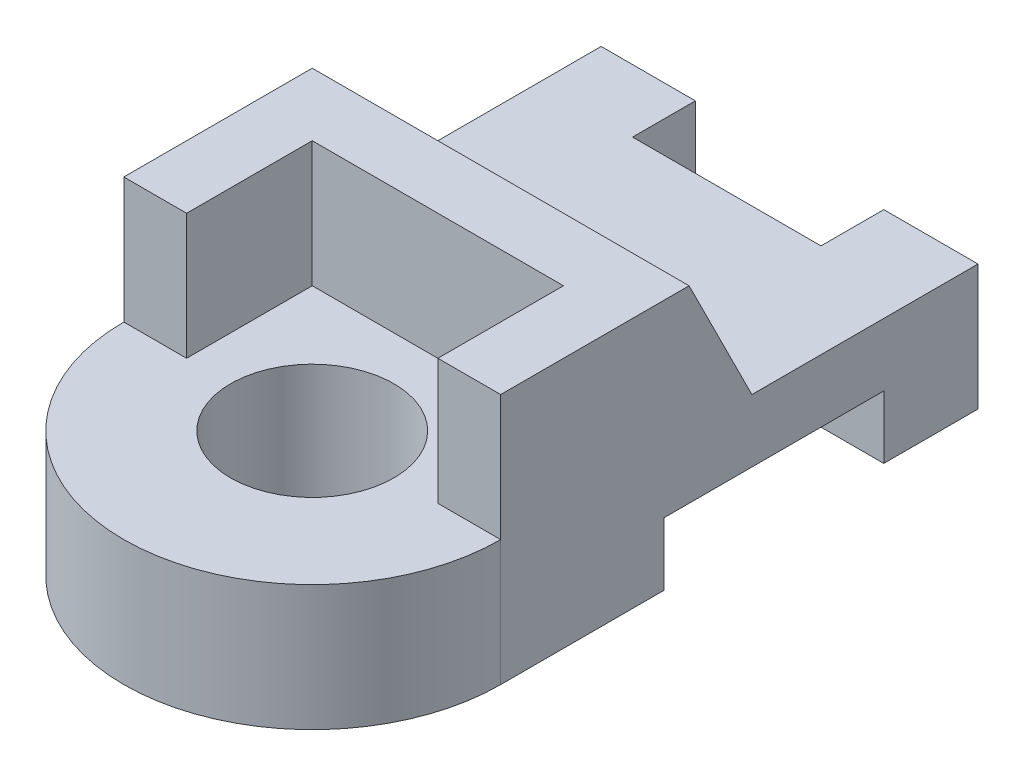
ISO-10303-21;
HEADER;
FILE_DESCRIPTION(('STEP AP214'),'2;1');
FILE_NAME('part.step','',(''),(''),'','','');
FILE_SCHEMA(('AUTOMOTIVE_DESIGN { 1 0 10303 214 1 1 1 1 }'));
ENDSEC;
DATA;
#1=APPLICATION_CONTEXT('core data for automotive mechanical design processes');
#2=APPLICATION_PROTOCOL_DEFINITION('international standard','automotive_design',2000,#1);
#3=PRODUCT_CONTEXT('',#1,'mechanical');
#4=PRODUCT('Part','Part','',(#3));
#5=PRODUCT_RELATED_PRODUCT_CATEGORY('part','',(#4));
#6=PRODUCT_DEFINITION_FORMATION('','',#4);
#7=PRODUCT_DEFINITION_CONTEXT('part definition',#1,'design');
#8=PRODUCT_DEFINITION('design','',#6,#7);
#9=PRODUCT_DEFINITION_SHAPE('','',#8);
#10=(LENGTH_UNIT() NAMED_UNIT(*) SI_UNIT(.MILLI.,.METRE.));
#11=(NAMED_UNIT(*) PLANE_ANGLE_UNIT() SI_UNIT($,.RADIAN.));
#12=(NAMED_UNIT(*) SI_UNIT($,.STERADIAN.) SOLID_ANGLE_UNIT());
#13=UNCERTAINTY_MEASURE_WITH_UNIT(LENGTH_MEASURE(1.E-05),#10,'distance_accuracy_value','');
#14=(GEOMETRIC_REPRESENTATION_CONTEXT(3) GLOBAL_UNCERTAINTY_ASSIGNED_CONTEXT((#13)) GLOBAL_UNIT_ASSIGNED_CONTEXT((#10,
#11,#12)) REPRESENTATION_CONTEXT('',''));
#15=CARTESIAN_POINT('',(0.,0.,0.));
#16=DIRECTION('',(0.,0.,1.));
#17=DIRECTION('',(1.,0.,0.));
#18=AXIS2_PLACEMENT_3D('',#15,#16,#17);
#19=CARTESIAN_POINT('',(30.,20.,0.));
#20=DIRECTION('',(0.,0.,-1.));
#21=DIRECTION('',(0.,1.,0.));
#22=AXIS2_PLACEMENT_3D('',#19,#20,#21);
#23=PLANE('',#22);
#24=DIRECTION('',(0.,1.,0.));
#25=VECTOR('',#24,1.);
#26=CARTESIAN_POINT('',(20.,-24.7213595499958,0.));
#27=LINE('',#26,#25);
#28=CARTESIAN_POINT('',(20.,20.,0.));
#29=VERTEX_POINT('',#28);
#30=CARTESIAN_POINT('',(20.,40.,0.));
#31=VERTEX_POINT('',#30);
#32=EDGE_CURVE('E193',#29,#31,#27,.T.);
#33=ORIENTED_EDGE('',*,*,#32,.F.);
#34=DIRECTION('',(-1.,0.,0.));
#35=VECTOR('',#34,1.);
#36=CARTESIAN_POINT('',(30.,20.,0.));
#37=LINE('',#36,#35);
#38=CARTESIAN_POINT('',(30.,20.,0.));
#39=VERTEX_POINT('',#38);
#40=EDGE_CURVE('E51',#39,#29,#37,.T.);
#41=ORIENTED_EDGE('',*,*,#40,.F.);
#42=DIRECTION('',(0.,-1.,0.));
#43=VECTOR('',#42,1.);
#44=CARTESIAN_POINT('',(30.,20.,0.));
#45=LINE('',#44,#43);
#46=CARTESIAN_POINT('',(30.,40.,0.));
#47=VERTEX_POINT('',#46);
#48=EDGE_CURVE('E201',#47,#39,#45,.T.);
#49=ORIENTED_EDGE('',*,*,#48,.F.);
#50=DIRECTION('',(-1.,0.,0.));
#51=VECTOR('',#50,1.);
#52=CARTESIAN_POINT('',(30.,40.,0.));
#53=LINE('',#52,#51);
#54=EDGE_CURVE('E196',#47,#31,#53,.T.);
#55=ORIENTED_EDGE('',*,*,#54,.T.);
#56=EDGE_LOOP('',(#33,#41,#49,#55));
#57=FACE_BOUND('',#56,.T.);
#58=ADVANCED_FACE('F41',(#57),#23,.F.);
#59=CARTESIAN_POINT('',(30.,40.,0.));
#60=DIRECTION('',(0.,-1.,0.));
#61=DIRECTION('',(0.,0.,-1.));
#62=AXIS2_PLACEMENT_3D('',#59,#60,#61);
#63=PLANE('',#62);
#64=DIRECTION('',(0.,0.,1.));
#65=VECTOR('',#64,1.);
#66=CARTESIAN_POINT('',(-20.,40.,0.));
#67=LINE('',#66,#65);
#68=CARTESIAN_POINT('',(-20.,40.,-20.));
#69=VERTEX_POINT('',#68);
#70=CARTESIAN_POINT('',(-20.,40.,0.));
#71=VERTEX_POINT('',#70);
#72=EDGE_CURVE('E173',#69,#71,#67,.T.);
#73=ORIENTED_EDGE('',*,*,#72,.F.);
#74=DIRECTION('',(-1.,0.,0.));
#75=VECTOR('',#74,1.);
#76=CARTESIAN_POINT('',(-20.,40.,-20.));
#77=LINE('',#76,#75);
#78=CARTESIAN_POINT('',(20.,40.,-20.));
#79=VERTEX_POINT('',#78);
#80=EDGE_CURVE('E195',#79,#69,#77,.T.);
#81=ORIENTED_EDGE('',*,*,#80,.F.);
#82=DIRECTION('',(0.,0.,-1.));
#83=VECTOR('',#82,1.);
#84=CARTESIAN_POINT('',(20.,40.,0.));
#85=LINE('',#84,#83);
#86=EDGE_CURVE('E59',#31,#79,#85,.T.);
#87=ORIENTED_EDGE('',*,*,#86,.F.);
#88=ORIENTED_EDGE('',*,*,#54,.F.);
#89=DIRECTION('',(0.,0.,1.));
#90=VECTOR('',#89,1.);
#91=CARTESIAN_POINT('',(30.,40.,0.));
#92=LINE('',#91,#90);
#93=CARTESIAN_POINT('',(30.,40.,-30.));
#94=VERTEX_POINT('',#93);
#95=EDGE_CURVE('E344',#94,#47,#92,.T.);
#96=ORIENTED_EDGE('',*,*,#95,.F.);
#97=DIRECTION('',(-1.,0.,0.));
#98=VECTOR('',#97,1.);
#99=CARTESIAN_POINT('',(30.,40.,-30.));
#100=LINE('',#99,#98);
#101=CARTESIAN_POINT('',(-30.,40.,-30.));
#102=VERTEX_POINT('',#101);
#103=EDGE_CURVE('E203',#94,#102,#100,.T.);
#104=ORIENTED_EDGE('',*,*,#103,.T.);
#105=DIRECTION('',(0.,0.,1.));
#106=VECTOR('',#105,1.);
#107=CARTESIAN_POINT('',(-30.,40.,0.));
#108=LINE('',#107,#106);
#109=CARTESIAN_POINT('',(-30.,40.,0.));
#110=VERTEX_POINT('',#109);
#111=EDGE_CURVE('E198',#102,#110,#108,.T.);
#112=ORIENTED_EDGE('',*,*,#111,.T.);
#113=EDGE_CURVE('E188',#71,#110,#53,.T.);
#114=ORIENTED_EDGE('',*,*,#113,.F.);
#115=EDGE_LOOP('',(#73,#81,#87,#88,#96,#104,#112,#114));
#116=FACE_BOUND('',#115,.T.);
#117=ADVANCED_FACE('F194',(#116),#63,.F.);
#118=CARTESIAN_POINT('',(0.,20.,0.));
#119=DIRECTION('',(0.,1.,0.));
#120=DIRECTION('',(0.,0.,1.));
#121=AXIS2_PLACEMENT_3D('',#118,#119,#120);
#122=PLANE('',#121);
#123=CARTESIAN_POINT('',(0.,20.,0.));
#124=DIRECTION('',(0.,1.,0.));
#125=DIRECTION('',(0.,0.,1.));
#126=AXIS2_PLACEMENT_3D('',#123,#124,#125);
#127=CIRCLE('',#126,13.);
#128=CARTESIAN_POINT('',(0.,20.,13.));
#129=VERTEX_POINT('',#128);
#130=EDGE_CURVE('E271',#129,#129,#127,.F.);
#131=ORIENTED_EDGE('',*,*,#130,.T.);
#132=EDGE_LOOP('',(#131));
#133=FACE_BOUND('',#132,.T.);
#134=CARTESIAN_POINT('',(0.,20.,0.));
#135=DIRECTION('',(0.,1.,0.));
#136=DIRECTION('',(0.,0.,1.));
#137=AXIS2_PLACEMENT_3D('',#134,#135,#136);
#138=CIRCLE('',#137,30.);
#139=CARTESIAN_POINT('',(-30.,20.,0.));
#140=VERTEX_POINT('',#139);
#141=EDGE_CURVE('E261',#39,#140,#138,.F.);
#142=ORIENTED_EDGE('',*,*,#141,.F.);
#143=ORIENTED_EDGE('',*,*,#40,.T.);
#144=DIRECTION('',(0.,0.,1.));
#145=VECTOR('',#144,1.);
#146=CARTESIAN_POINT('',(20.,20.,0.));
#147=LINE('',#146,#145);
#148=CARTESIAN_POINT('',(20.,20.,-20.));
#149=VERTEX_POINT('',#148);
#150=EDGE_CURVE('E359',#149,#29,#147,.T.);
#151=ORIENTED_EDGE('',*,*,#150,.F.);
#152=DIRECTION('',(1.,0.,0.));
#153=VECTOR('',#152,1.);
#154=CARTESIAN_POINT('',(-20.,20.,-20.));
#155=LINE('',#154,#153);
#156=CARTESIAN_POINT('',(-20.,20.,-20.));
#157=VERTEX_POINT('',#156);
#158=EDGE_CURVE('E363',#157,#149,#155,.T.);
#159=ORIENTED_EDGE('',*,*,#158,.F.);
#160=DIRECTION('',(0.,0.,-1.));
#161=VECTOR('',#160,1.);
#162=CARTESIAN_POINT('',(-20.,20.,0.));
#163=LINE('',#162,#161);
#164=CARTESIAN_POINT('',(-20.,20.,0.));
#165=VERTEX_POINT('',#164);
#166=EDGE_CURVE('E357',#165,#157,#163,.T.);
#167=ORIENTED_EDGE('',*,*,#166,.F.);
#168=EDGE_CURVE('E11',#165,#140,#37,.T.);
#169=ORIENTED_EDGE('',*,*,#168,.T.);
#170=EDGE_LOOP('',(#142,#143,#151,#159,#167,#169));
#171=FACE_BOUND('',#170,.T.);
#172=ADVANCED_FACE('F360',(#133,#171),#122,.T.);
#173=CARTESIAN_POINT('',(0.,20.,-76.));
#174=DIRECTION('',(0.,0.,1.));
#175=DIRECTION('',(1.,0.,0.));
#176=AXIS2_PLACEMENT_3D('',#173,#174,#175);
#177=PLANE('',#176);
#178=DIRECTION('',(0.,1.,0.));
#179=VECTOR('',#178,1.);
#180=CARTESIAN_POINT('',(-15.,-0.001000000000001,-76.));
#181=LINE('',#180,#179);
#182=CARTESIAN_POINT('',(-15.,0.,-76.));
#183=VERTEX_POINT('',#182);
#184=CARTESIAN_POINT('',(-15.,20.,-76.));
#185=VERTEX_POINT('',#184);
#186=EDGE_CURVE('E222',#183,#185,#181,.T.);
#187=ORIENTED_EDGE('',*,*,#186,.F.);
#188=DIRECTION('',(-1.,0.,0.));
#189=VECTOR('',#188,1.);
#190=CARTESIAN_POINT('',(0.,0.,-76.));
#191=LINE('',#190,#189);
#192=CARTESIAN_POINT('',(-30.,0.,-76.));
#193=VERTEX_POINT('',#192);
#194=EDGE_CURVE('E285',#183,#193,#191,.T.);
#195=ORIENTED_EDGE('',*,*,#194,.T.);
#196=DIRECTION('',(0.,-1.,0.));
#197=VECTOR('',#196,1.);
#198=CARTESIAN_POINT('',(-30.,20.,-76.));
#199=LINE('',#198,#197);
#200=CARTESIAN_POINT('',(-30.,20.,-76.));
#201=VERTEX_POINT('',#200);
#202=EDGE_CURVE('E273',#201,#193,#199,.T.);
#203=ORIENTED_EDGE('',*,*,#202,.F.);
#204=DIRECTION('',(-1.,0.,0.));
#205=VECTOR('',#204,1.);
#206=CARTESIAN_POINT('',(0.,20.,-76.));
#207=LINE('',#206,#205);
#208=EDGE_CURVE('E270',#185,#201,#207,.T.);
#209=ORIENTED_EDGE('',*,*,#208,.F.);
#210=EDGE_LOOP('',(#187,#195,#203,#209));
#211=FACE_BOUND('',#210,.T.);
#212=ADVANCED_FACE('F430',(#211),#177,.F.);
#213=CARTESIAN_POINT('',(0.,0.,0.));
#214=DIRECTION('',(0.,1.,0.));
#215=DIRECTION('',(0.,0.,1.));
#216=AXIS2_PLACEMENT_3D('',#213,#214,#215);
#217=PLANE('',#216);
#218=DIRECTION('',(0.,0.,-1.));
#219=VECTOR('',#218,1.);
#220=CARTESIAN_POINT('',(-15.,0.,-76.));
#221=LINE('',#220,#219);
#222=CARTESIAN_POINT('',(-15.,0.,-66.));
#223=VERTEX_POINT('',#222);
#224=EDGE_CURVE('E211',#223,#183,#221,.T.);
#225=ORIENTED_EDGE('',*,*,#224,.F.);
#226=DIRECTION('',(-1.,0.,0.));
#227=VECTOR('',#226,1.);
#228=CARTESIAN_POINT('',(-15.,0.,-66.));
#229=LINE('',#228,#227);
#230=CARTESIAN_POINT('',(15.,0.,-66.));
#231=VERTEX_POINT('',#230);
#232=EDGE_CURVE('E224',#231,#223,#229,.T.);
#233=ORIENTED_EDGE('',*,*,#232,.F.);
#234=DIRECTION('',(0.,0.,1.));
#235=VECTOR('',#234,1.);
#236=CARTESIAN_POINT('',(15.,0.,-76.));
#237=LINE('',#236,#235);
#238=CARTESIAN_POINT('',(15.,0.,-76.));
#239=VERTEX_POINT('',#238);
#240=EDGE_CURVE('E208',#239,#231,#237,.T.);
#241=ORIENTED_EDGE('',*,*,#240,.F.);
#242=CARTESIAN_POINT('',(30.,0.,-76.));
#243=VERTEX_POINT('',#242);
#244=EDGE_CURVE('E288',#243,#239,#191,.T.);
#245=ORIENTED_EDGE('',*,*,#244,.F.);
#246=DIRECTION('',(0.,0.,-1.));
#247=VECTOR('',#246,1.);
#248=CARTESIAN_POINT('',(30.,0.,0.));
#249=LINE('',#248,#247);
#250=CARTESIAN_POINT('',(30.,0.,-61.));
#251=VERTEX_POINT('',#250);
#252=EDGE_CURVE('E281',#251,#243,#249,.T.);
#253=ORIENTED_EDGE('',*,*,#252,.F.);
#254=DIRECTION('',(1.,0.,0.));
#255=VECTOR('',#254,1.);
#256=CARTESIAN_POINT('',(-30.001,0.,-61.));
#257=LINE('',#256,#255);
#258=CARTESIAN_POINT('',(-30.,0.,-61.));
#259=VERTEX_POINT('',#258);
#260=EDGE_CURVE('E254',#259,#251,#257,.T.);
#261=ORIENTED_EDGE('',*,*,#260,.F.);
#262=DIRECTION('',(0.,0.,1.));
#263=VECTOR('',#262,1.);
#264=CARTESIAN_POINT('',(-30.,0.,0.));
#265=LINE('',#264,#263);
#266=EDGE_CURVE('E274',#193,#259,#265,.T.);
#267=ORIENTED_EDGE('',*,*,#266,.F.);
#268=ORIENTED_EDGE('',*,*,#194,.F.);
#269=EDGE_LOOP('',(#225,#233,#241,#245,#253,#261,#267,#268));
#270=FACE_BOUND('',#269,.T.);
#271=ADVANCED_FACE('F328',(#270),#217,.F.);
#272=CARTESIAN_POINT('',(-30.,20.,0.));
#273=DIRECTION('',(1.,0.,0.));
#274=DIRECTION('',(0.,0.,-1.));
#275=AXIS2_PLACEMENT_3D('',#272,#273,#274);
#276=PLANE('',#275);
#277=DIRECTION('',(0.,1.,0.));
#278=VECTOR('',#277,1.);
#279=CARTESIAN_POINT('',(-30.,0.,-26.));
#280=LINE('',#279,#278);
#281=CARTESIAN_POINT('',(-30.,0.,-26.));
#282=VERTEX_POINT('',#281);
#283=CARTESIAN_POINT('',(-30.,10.,-26.));
#284=VERTEX_POINT('',#283);
#285=EDGE_CURVE('E236',#282,#284,#280,.T.);
#286=ORIENTED_EDGE('',*,*,#285,.F.);
#287=CARTESIAN_POINT('',(-30.,0.,0.));
#288=VERTEX_POINT('',#287);
#289=EDGE_CURVE('E253',#282,#288,#265,.T.);
#290=ORIENTED_EDGE('',*,*,#289,.T.);
#291=DIRECTION('',(0.,-1.,0.));
#292=VECTOR('',#291,1.);
#293=CARTESIAN_POINT('',(-30.,20.,0.));
#294=LINE('',#293,#292);
#295=EDGE_CURVE('E44',#140,#288,#294,.T.);
#296=ORIENTED_EDGE('',*,*,#295,.F.);
#297=DIRECTION('',(0.,-1.,0.));
#298=VECTOR('',#297,1.);
#299=CARTESIAN_POINT('',(-30.,20.,0.));
#300=LINE('',#299,#298);
#301=EDGE_CURVE('E342',#110,#140,#300,.T.);
#302=ORIENTED_EDGE('',*,*,#301,.F.);
#303=ORIENTED_EDGE('',*,*,#111,.F.);
#304=DIRECTION('',(0.,0.894427190999916,0.447213595499959));
#305=VECTOR('',#304,1.);
#306=CARTESIAN_POINT('',(-30.,40.,-30.));
#307=LINE('',#306,#305);
#308=CARTESIAN_POINT('',(-30.,20.,-40.));
#309=VERTEX_POINT('',#308);
#310=EDGE_CURVE('E362',#309,#102,#307,.T.);
#311=ORIENTED_EDGE('',*,*,#310,.F.);
#312=DIRECTION('',(0.,0.,1.));
#313=VECTOR('',#312,1.);
#314=CARTESIAN_POINT('',(-30.,20.,0.));
#315=LINE('',#314,#313);
#316=EDGE_CURVE('E259',#201,#309,#315,.T.);
#317=ORIENTED_EDGE('',*,*,#316,.F.);
#318=ORIENTED_EDGE('',*,*,#202,.T.);
#319=ORIENTED_EDGE('',*,*,#266,.T.);
#320=DIRECTION('',(0.,-1.,0.));
#321=VECTOR('',#320,1.);
#322=CARTESIAN_POINT('',(-30.,0.,-61.));
#323=LINE('',#322,#321);
#324=CARTESIAN_POINT('',(-30.,10.,-61.));
#325=VERTEX_POINT('',#324);
#326=EDGE_CURVE('E231',#325,#259,#323,.T.);
#327=ORIENTED_EDGE('',*,*,#326,.F.);
#328=DIRECTION('',(0.,0.,-1.));
#329=VECTOR('',#328,1.);
#330=CARTESIAN_POINT('',(-30.,10.,-26.));
#331=LINE('',#330,#329);
#332=EDGE_CURVE('E232',#284,#325,#331,.T.);
#333=ORIENTED_EDGE('',*,*,#332,.F.);
#334=EDGE_LOOP('',(#286,#290,#296,#302,#303,#311,#317,#318,#319,#327,#333));
#335=FACE_BOUND('',#334,.T.);
#336=ADVANCED_FACE('F43',(#335),#276,.F.);
#337=CARTESIAN_POINT('',(30.,20.,0.));
#338=DIRECTION('',(-1.,0.,0.));
#339=DIRECTION('',(0.,0.,1.));
#340=AXIS2_PLACEMENT_3D('',#337,#338,#339);
#341=PLANE('',#340);
#342=DIRECTION('',(0.,-1.,0.));
#343=VECTOR('',#342,1.);
#344=CARTESIAN_POINT('',(30.,0.,-26.));
#345=LINE('',#344,#343);
#346=CARTESIAN_POINT('',(30.,10.,-26.));
#347=VERTEX_POINT('',#346);
#348=CARTESIAN_POINT('',(30.,0.,-26.));
#349=VERTEX_POINT('',#348);
#350=EDGE_CURVE('E241',#347,#349,#345,.T.);
#351=ORIENTED_EDGE('',*,*,#350,.F.);
#352=DIRECTION('',(0.,0.,1.));
#353=VECTOR('',#352,1.);
#354=CARTESIAN_POINT('',(30.,10.,-26.));
#355=LINE('',#354,#353);
#356=CARTESIAN_POINT('',(30.,10.,-61.));
#357=VERTEX_POINT('',#356);
#358=EDGE_CURVE('E245',#357,#347,#355,.T.);
#359=ORIENTED_EDGE('',*,*,#358,.F.);
#360=DIRECTION('',(0.,1.,0.));
#361=VECTOR('',#360,1.);
#362=CARTESIAN_POINT('',(30.,0.,-61.));
#363=LINE('',#362,#361);
#364=EDGE_CURVE('E244',#251,#357,#363,.T.);
#365=ORIENTED_EDGE('',*,*,#364,.F.);
#366=ORIENTED_EDGE('',*,*,#252,.T.);
#367=DIRECTION('',(0.,-1.,0.));
#368=VECTOR('',#367,1.);
#369=CARTESIAN_POINT('',(30.,20.,-76.));
#370=LINE('',#369,#368);
#371=CARTESIAN_POINT('',(30.,20.,-76.));
#372=VERTEX_POINT('',#371);
#373=EDGE_CURVE('E291',#372,#243,#370,.T.);
#374=ORIENTED_EDGE('',*,*,#373,.F.);
#375=DIRECTION('',(0.,0.,-1.));
#376=VECTOR('',#375,1.);
#377=CARTESIAN_POINT('',(30.,20.,0.));
#378=LINE('',#377,#376);
#379=CARTESIAN_POINT('',(30.,20.,-40.));
#380=VERTEX_POINT('',#379);
#381=EDGE_CURVE('E264',#380,#372,#378,.T.);
#382=ORIENTED_EDGE('',*,*,#381,.F.);
#383=DIRECTION('',(0.,0.894427190999916,0.447213595499959));
#384=VECTOR('',#383,1.);
#385=CARTESIAN_POINT('',(30.,40.,-30.));
#386=LINE('',#385,#384);
#387=EDGE_CURVE('E337',#380,#94,#386,.T.);
#388=ORIENTED_EDGE('',*,*,#387,.T.);
#389=ORIENTED_EDGE('',*,*,#95,.T.);
#390=ORIENTED_EDGE('',*,*,#48,.T.);
#391=DIRECTION('',(0.,-1.,0.));
#392=VECTOR('',#391,1.);
#393=CARTESIAN_POINT('',(30.,20.,0.));
#394=LINE('',#393,#392);
#395=CARTESIAN_POINT('',(30.,0.,0.));
#396=VERTEX_POINT('',#395);
#397=EDGE_CURVE('E293',#39,#396,#394,.T.);
#398=ORIENTED_EDGE('',*,*,#397,.T.);
#399=EDGE_CURVE('E282',#396,#349,#249,.T.);
#400=ORIENTED_EDGE('',*,*,#399,.T.);
#401=EDGE_LOOP('',(#351,#359,#365,#366,#374,#382,#388,#389,#390,#398,#400));
#402=FACE_BOUND('',#401,.T.);
#403=ADVANCED_FACE('F313',(#402),#341,.F.);
#404=CARTESIAN_POINT('',(0.,20.,0.));
#405=DIRECTION('',(0.,-1.,0.));
#406=DIRECTION('',(0.,0.,-1.));
#407=AXIS2_PLACEMENT_3D('',#404,#405,#406);
#408=CYLINDRICAL_SURFACE('',#407,30.);
#409=CARTESIAN_POINT('',(0.,0.,0.));
#410=DIRECTION('',(0.,1.,0.));
#411=DIRECTION('',(0.,0.,1.));
#412=AXIS2_PLACEMENT_3D('',#409,#410,#411);
#413=CIRCLE('',#412,30.);
#414=EDGE_CURVE('E279',#396,#288,#413,.F.);
#415=ORIENTED_EDGE('',*,*,#414,.F.);
#416=ORIENTED_EDGE('',*,*,#397,.F.);
#417=ORIENTED_EDGE('',*,*,#141,.T.);
#418=ORIENTED_EDGE('',*,*,#295,.T.);
#419=EDGE_LOOP('',(#415,#416,#417,#418));
#420=FACE_BOUND('',#419,.T.);
#421=ADVANCED_FACE('F301',(#420),#408,.T.);
#422=ORIENTED_EDGE('',*,*,#244,.T.);
#423=DIRECTION('',(0.,1.,0.));
#424=VECTOR('',#423,1.);
#425=CARTESIAN_POINT('',(15.,-0.001000000000001,-76.));
#426=LINE('',#425,#424);
#427=CARTESIAN_POINT('',(15.,20.,-76.));
#428=VERTEX_POINT('',#427);
#429=EDGE_CURVE('E221',#239,#428,#426,.T.);
#430=ORIENTED_EDGE('',*,*,#429,.T.);
#431=EDGE_CURVE('E268',#372,#428,#207,.T.);
#432=ORIENTED_EDGE('',*,*,#431,.F.);
#433=ORIENTED_EDGE('',*,*,#373,.T.);
#434=EDGE_LOOP('',(#422,#430,#432,#433));
#435=FACE_BOUND('',#434,.T.);
#436=ADVANCED_FACE('F331',(#435),#177,.F.);
#437=CARTESIAN_POINT('',(0.,20.,0.));
#438=DIRECTION('',(0.,-1.,0.));
#439=DIRECTION('',(0.,0.,-1.));
#440=AXIS2_PLACEMENT_3D('',#437,#438,#439);
#441=CYLINDRICAL_SURFACE('',#440,13.);
#442=ORIENTED_EDGE('',*,*,#130,.F.);
#443=EDGE_LOOP('',(#442));
#444=FACE_BOUND('',#443,.T.);
#445=CARTESIAN_POINT('',(0.,0.,0.));
#446=DIRECTION('',(0.,1.,0.));
#447=DIRECTION('',(0.,0.,1.));
#448=AXIS2_PLACEMENT_3D('',#445,#446,#447);
#449=CIRCLE('',#448,13.);
#450=CARTESIAN_POINT('',(0.,0.,13.));
#451=VERTEX_POINT('',#450);
#452=EDGE_CURVE('E265',#451,#451,#449,.F.);
#453=ORIENTED_EDGE('',*,*,#452,.T.);
#454=EDGE_LOOP('',(#453));
#455=FACE_BOUND('',#454,.T.);
#456=ADVANCED_FACE('F419',(#444,#455),#441,.F.);
#457=DIRECTION('',(-1.,0.,0.));
#458=VECTOR('',#457,1.);
#459=CARTESIAN_POINT('',(30.,20.,-40.));
#460=LINE('',#459,#458);
#461=EDGE_CURVE('E68',#380,#309,#460,.T.);
#462=ORIENTED_EDGE('',*,*,#461,.F.);
#463=ORIENTED_EDGE('',*,*,#381,.T.);
#464=ORIENTED_EDGE('',*,*,#431,.T.);
#465=DIRECTION('',(0.,0.,-1.));
#466=VECTOR('',#465,1.);
#467=CARTESIAN_POINT('',(15.,20.,-76.));
#468=LINE('',#467,#466);
#469=CARTESIAN_POINT('',(15.,20.,-66.));
#470=VERTEX_POINT('',#469);
#471=EDGE_CURVE('E217',#470,#428,#468,.T.);
#472=ORIENTED_EDGE('',*,*,#471,.F.);
#473=DIRECTION('',(1.,0.,0.));
#474=VECTOR('',#473,1.);
#475=CARTESIAN_POINT('',(-15.,20.,-66.));
#476=LINE('',#475,#474);
#477=CARTESIAN_POINT('',(-15.,20.,-66.));
#478=VERTEX_POINT('',#477);
#479=EDGE_CURVE('E214',#478,#470,#476,.T.);
#480=ORIENTED_EDGE('',*,*,#479,.F.);
#481=DIRECTION('',(0.,0.,1.));
#482=VECTOR('',#481,1.);
#483=CARTESIAN_POINT('',(-15.,20.,-76.));
#484=LINE('',#483,#482);
#485=EDGE_CURVE('E213',#185,#478,#484,.T.);
#486=ORIENTED_EDGE('',*,*,#485,.F.);
#487=ORIENTED_EDGE('',*,*,#208,.T.);
#488=ORIENTED_EDGE('',*,*,#316,.T.);
#489=EDGE_LOOP('',(#462,#463,#464,#472,#480,#486,#487,#488));
#490=FACE_BOUND('',#489,.T.);
#491=ADVANCED_FACE('F416',(#490),#122,.T.);
#492=ORIENTED_EDGE('',*,*,#289,.F.);
#493=DIRECTION('',(1.,0.,0.));
#494=VECTOR('',#493,1.);
#495=CARTESIAN_POINT('',(-30.001,0.,-26.));
#496=LINE('',#495,#494);
#497=EDGE_CURVE('E246',#282,#349,#496,.T.);
#498=ORIENTED_EDGE('',*,*,#497,.T.);
#499=ORIENTED_EDGE('',*,*,#399,.F.);
#500=ORIENTED_EDGE('',*,*,#414,.T.);
#501=EDGE_LOOP('',(#492,#498,#499,#500));
#502=FACE_BOUND('',#501,.T.);
#503=ORIENTED_EDGE('',*,*,#452,.F.);
#504=EDGE_LOOP('',(#503));
#505=FACE_BOUND('',#504,.T.);
#506=ADVANCED_FACE('F306',(#502,#505),#217,.F.);
#507=CARTESIAN_POINT('',(-30.001,0.,-26.));
#508=DIRECTION('',(0.,0.,1.));
#509=DIRECTION('',(1.,0.,0.));
#510=AXIS2_PLACEMENT_3D('',#507,#508,#509);
#511=PLANE('',#510);
#512=ORIENTED_EDGE('',*,*,#285,.T.);
#513=DIRECTION('',(1.,0.,0.));
#514=VECTOR('',#513,1.);
#515=CARTESIAN_POINT('',(-30.001,10.,-26.));
#516=LINE('',#515,#514);
#517=EDGE_CURVE('E249',#284,#347,#516,.T.);
#518=ORIENTED_EDGE('',*,*,#517,.T.);
#519=ORIENTED_EDGE('',*,*,#350,.T.);
#520=ORIENTED_EDGE('',*,*,#497,.F.);
#521=EDGE_LOOP('',(#512,#518,#519,#520));
#522=FACE_BOUND('',#521,.T.);
#523=ADVANCED_FACE('F312',(#522),#511,.F.);
#524=CARTESIAN_POINT('',(-30.001,10.,-26.));
#525=DIRECTION('',(0.,1.,0.));
#526=DIRECTION('',(0.,0.,1.));
#527=AXIS2_PLACEMENT_3D('',#524,#525,#526);
#528=PLANE('',#527);
#529=ORIENTED_EDGE('',*,*,#332,.T.);
#530=DIRECTION('',(1.,0.,0.));
#531=VECTOR('',#530,1.);
#532=CARTESIAN_POINT('',(-30.001,10.,-61.));
#533=LINE('',#532,#531);
#534=EDGE_CURVE('E252',#325,#357,#533,.T.);
#535=ORIENTED_EDGE('',*,*,#534,.T.);
#536=ORIENTED_EDGE('',*,*,#358,.T.);
#537=ORIENTED_EDGE('',*,*,#517,.F.);
#538=EDGE_LOOP('',(#529,#535,#536,#537));
#539=FACE_BOUND('',#538,.T.);
#540=ADVANCED_FACE('F317',(#539),#528,.F.);
#541=CARTESIAN_POINT('',(-30.001,0.,-61.));
#542=DIRECTION('',(0.,0.,-1.));
#543=DIRECTION('',(-1.,0.,0.));
#544=AXIS2_PLACEMENT_3D('',#541,#542,#543);
#545=PLANE('',#544);
#546=ORIENTED_EDGE('',*,*,#326,.T.);
#547=ORIENTED_EDGE('',*,*,#260,.T.);
#548=ORIENTED_EDGE('',*,*,#364,.T.);
#549=ORIENTED_EDGE('',*,*,#534,.F.);
#550=EDGE_LOOP('',(#546,#547,#548,#549));
#551=FACE_BOUND('',#550,.T.);
#552=ADVANCED_FACE('F325',(#551),#545,.F.);
#553=CARTESIAN_POINT('',(-15.,-0.001000000000001,-76.));
#554=DIRECTION('',(-1.,0.,0.));
#555=DIRECTION('',(0.,0.,1.));
#556=AXIS2_PLACEMENT_3D('',#553,#554,#555);
#557=PLANE('',#556);
#558=ORIENTED_EDGE('',*,*,#224,.T.);
#559=ORIENTED_EDGE('',*,*,#186,.T.);
#560=ORIENTED_EDGE('',*,*,#485,.T.);
#561=DIRECTION('',(0.,1.,0.));
#562=VECTOR('',#561,1.);
#563=CARTESIAN_POINT('',(-15.,-0.001000000000001,-66.));
#564=LINE('',#563,#562);
#565=EDGE_CURVE('E219',#223,#478,#564,.T.);
#566=ORIENTED_EDGE('',*,*,#565,.F.);
#567=EDGE_LOOP('',(#558,#559,#560,#566));
#568=FACE_BOUND('',#567,.T.);
#569=ADVANCED_FACE('F406',(#568),#557,.F.);
#570=CARTESIAN_POINT('',(15.,-0.001000000000001,-76.));
#571=DIRECTION('',(1.,0.,0.));
#572=DIRECTION('',(0.,0.,-1.));
#573=AXIS2_PLACEMENT_3D('',#570,#571,#572);
#574=PLANE('',#573);
#575=ORIENTED_EDGE('',*,*,#240,.T.);
#576=DIRECTION('',(0.,1.,0.));
#577=VECTOR('',#576,1.);
#578=CARTESIAN_POINT('',(15.,-0.001000000000001,-66.));
#579=LINE('',#578,#577);
#580=EDGE_CURVE('E227',#231,#470,#579,.T.);
#581=ORIENTED_EDGE('',*,*,#580,.T.);
#582=ORIENTED_EDGE('',*,*,#471,.T.);
#583=ORIENTED_EDGE('',*,*,#429,.F.);
#584=EDGE_LOOP('',(#575,#581,#582,#583));
#585=FACE_BOUND('',#584,.T.);
#586=ADVANCED_FACE('F402',(#585),#574,.F.);
#587=CARTESIAN_POINT('',(-15.,-0.001000000000001,-66.));
#588=DIRECTION('',(0.,0.,1.));
#589=DIRECTION('',(1.,0.,0.));
#590=AXIS2_PLACEMENT_3D('',#587,#588,#589);
#591=PLANE('',#590);
#592=ORIENTED_EDGE('',*,*,#232,.T.);
#593=ORIENTED_EDGE('',*,*,#565,.T.);
#594=ORIENTED_EDGE('',*,*,#479,.T.);
#595=ORIENTED_EDGE('',*,*,#580,.F.);
#596=EDGE_LOOP('',(#592,#593,#594,#595));
#597=FACE_BOUND('',#596,.T.);
#598=ADVANCED_FACE('F395',(#597),#591,.F.);
#599=CARTESIAN_POINT('',(30.,40.,-30.));
#600=DIRECTION('',(0.,-0.447213595499958,0.894427190999916));
#601=DIRECTION('',(0.,-0.894427190999916,-0.447213595499959));
#602=AXIS2_PLACEMENT_3D('',#599,#600,#601);
#603=PLANE('',#602);
#604=ORIENTED_EDGE('',*,*,#461,.T.);
#605=ORIENTED_EDGE('',*,*,#310,.T.);
#606=ORIENTED_EDGE('',*,*,#103,.F.);
#607=ORIENTED_EDGE('',*,*,#387,.F.);
#608=EDGE_LOOP('',(#604,#605,#606,#607));
#609=FACE_BOUND('',#608,.T.);
#610=ADVANCED_FACE('F340',(#609),#603,.F.);
#611=ORIENTED_EDGE('',*,*,#168,.F.);
#612=DIRECTION('',(0.,1.,0.));
#613=VECTOR('',#612,1.);
#614=CARTESIAN_POINT('',(-20.,-24.7213595499958,0.));
#615=LINE('',#614,#613);
#616=EDGE_CURVE('E180',#165,#71,#615,.T.);
#617=ORIENTED_EDGE('',*,*,#616,.T.);
#618=ORIENTED_EDGE('',*,*,#113,.T.);
#619=ORIENTED_EDGE('',*,*,#301,.T.);
#620=EDGE_LOOP('',(#611,#617,#618,#619));
#621=FACE_BOUND('',#620,.T.);
#622=ADVANCED_FACE('F187',(#621),#23,.F.);
#623=CARTESIAN_POINT('',(-20.,-24.7213595499958,0.));
#624=DIRECTION('',(-1.,0.,0.));
#625=DIRECTION('',(0.,0.,1.));
#626=AXIS2_PLACEMENT_3D('',#623,#624,#625);
#627=PLANE('',#626);
#628=ORIENTED_EDGE('',*,*,#166,.T.);
#629=DIRECTION('',(0.,1.,0.));
#630=VECTOR('',#629,1.);
#631=CARTESIAN_POINT('',(-20.,-24.7213595499958,-20.));
#632=LINE('',#631,#630);
#633=EDGE_CURVE('E177',#157,#69,#632,.T.);
#634=ORIENTED_EDGE('',*,*,#633,.T.);
#635=ORIENTED_EDGE('',*,*,#72,.T.);
#636=ORIENTED_EDGE('',*,*,#616,.F.);
#637=EDGE_LOOP('',(#628,#634,#635,#636));
#638=FACE_BOUND('',#637,.T.);
#639=ADVANCED_FACE('F178',(#638),#627,.F.);
#640=CARTESIAN_POINT('',(-20.,-24.7213595499958,-20.));
#641=DIRECTION('',(0.,0.,-1.));
#642=DIRECTION('',(-1.,0.,0.));
#643=AXIS2_PLACEMENT_3D('',#640,#641,#642);
#644=PLANE('',#643);
#645=ORIENTED_EDGE('',*,*,#158,.T.);
#646=DIRECTION('',(0.,1.,0.));
#647=VECTOR('',#646,1.);
#648=CARTESIAN_POINT('',(20.,-24.7213595499958,-20.));
#649=LINE('',#648,#647);
#650=EDGE_CURVE('E371',#149,#79,#649,.T.);
#651=ORIENTED_EDGE('',*,*,#650,.T.);
#652=ORIENTED_EDGE('',*,*,#80,.T.);
#653=ORIENTED_EDGE('',*,*,#633,.F.);
#654=EDGE_LOOP('',(#645,#651,#652,#653));
#655=FACE_BOUND('',#654,.T.);
#656=ADVANCED_FACE('F374',(#655),#644,.F.);
#657=CARTESIAN_POINT('',(20.,-24.7213595499958,0.));
#658=DIRECTION('',(1.,0.,0.));
#659=DIRECTION('',(0.,0.,-1.));
#660=AXIS2_PLACEMENT_3D('',#657,#658,#659);
#661=PLANE('',#660);
#662=ORIENTED_EDGE('',*,*,#150,.T.);
#663=ORIENTED_EDGE('',*,*,#32,.T.);
#664=ORIENTED_EDGE('',*,*,#86,.T.);
#665=ORIENTED_EDGE('',*,*,#650,.F.);
#666=EDGE_LOOP('',(#662,#663,#664,#665));
#667=FACE_BOUND('',#666,.T.);
#668=ADVANCED_FACE('F373',(#667),#661,.F.);
#669=CLOSED_SHELL('',(#58,#117,#172,#212,#271,#336,#403,#421,#436,#456,#491,#506,#523,#540,#552,
#569,#586,#598,#610,#622,#639,#656,#668));
#670=MANIFOLD_SOLID_BREP('B2',#669);
#671=ADVANCED_BREP_SHAPE_REPRESENTATION('',(#18,#670),#14);
#672=SHAPE_DEFINITION_REPRESENTATION(#9,#671);
ENDSEC;
END-ISO-10303-21;
